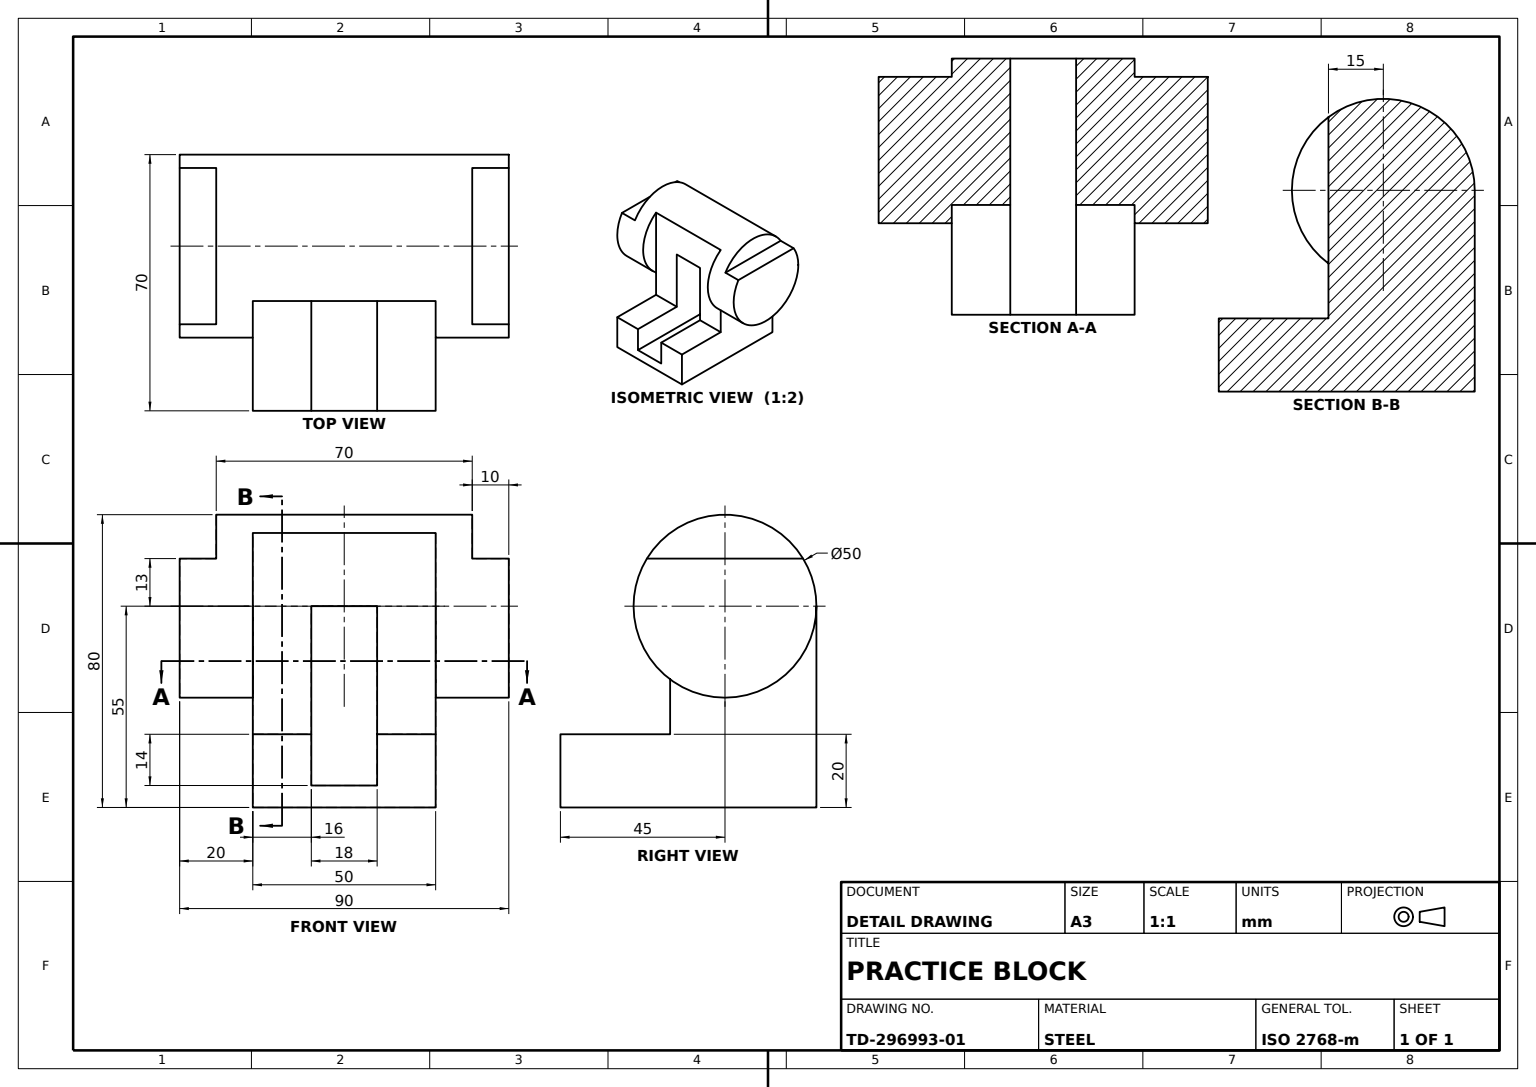
from build123d import *
from build123d.topology import SkipClean

# Parameters (mm, degrees)
U_BASE_DEPTH             = 20
UPRIGHT_WEB_DEPTH        = 50
CYLINDER_50_SKETCH_R     = 25
CYLINDER_50_DEPTH        = 50
WEB_CLEARANCE_CUT_DEPTH  = 50
SIDE_RELIEF_CUT_SKETCH_W = 18
SIDE_RELIEF_CUT_SKETCH_H = 35
SIDE_RELIEF_CUT_DEPTH    = 50
BASE_SLOT_CUT_SKETCH_W   = 50
BASE_SLOT_CUT_SKETCH_H   = 50
BASE_SLOT_CUT_DEPTH      = 10
WEB_SLOT_CUT_SKETCH_W    = 5
WEB_SLOT_CUT_SKETCH_H    = 50
WEB_SLOT_CUT_DEPTH       = 10
END_START                = 20
END_BOSS_A_SKETCH_R      = 25
END_BOSS_A_50_DEPTH      = 20
END_BOSS_B_SKETCH_R      = 25
END_BOSS_B_50_DEPTH      = 20
END_SLOT_A_DEPTH         = 10
END_START_2              = -10
END_SLOT_B_DEPTH         = 10


with BuildPart() as part:
    # U Base Profile Sketch → U Base (new body)
    with BuildSketch(Plane(origin=(0, 0, 0), x_dir=(0, 0, -1), z_dir=(1, 0, 0))):
        Polygon((25, 0), (-25, 0), (-25, 20), (-9, 20), (-9, 6), (9, 6), (9, 20), (25, 20), align=None)
    extrude(amount=U_BASE_DEPTH)

    # Upright Web Sketch → Upright Web (add)
    with BuildSketch(Plane.ZY):
        Polygon((-9, 20), (-9, 65), (9, 65), (9, 20), (25, 20), (25, 70), (-25, 70), (-25, 20), align=None)
        Polygon((25, 20), (9, 20), (9, 6), (-9, 6), (-9, 20), (-25, 20), (-25, 0), (25, 0), align=None)
    extrude(amount=UPRIGHT_WEB_DEPTH)

    # Cylinder Ø50 Sketch → Cylinder Ø50 (add)
    with BuildSketch(Plane.XY.offset(25)):
        with Locations((-25, 55)):
            Circle(CYLINDER_50_SKETCH_R)
    extrude(amount=-CYLINDER_50_DEPTH)

    # Web Clearance Cut Sketch → Web Clearance Cut (cut)
    with SkipClean():  # the faces are left unmerged after this step: merging them gives an invalid solid
        with BuildSketch(Plane.XY.offset(25)):
            with BuildLine():
                Line((-50, 70), (-50, 55))
                ThreePointArc((-50, 55), (-48.717082, 62.905694), (-45, 70))
                Line((-45, 70), (-50, 70))
            make_face()
            with BuildLine():
                ThreePointArc((-5, 70), (-1.282918, 62.905694), (0, 55))
                Line((0, 55), (0, 70))
                Line((0, 70), (-5, 70))
            make_face()
        extrude(amount=-WEB_CLEARANCE_CUT_DEPTH, mode=Mode.SUBTRACT)

    # Side Relief Cut Sketch → Side Relief Cut (cut)
    with SkipClean():  # the faces are left unmerged after this step: merging them gives an invalid solid
        with BuildSketch(Plane(origin=(0, 0, 0), x_dir=(0, 0, -1), z_dir=(1, 0, 0))):
            with Locations((0, 37.5)):
                Rectangle(SIDE_RELIEF_CUT_SKETCH_W, SIDE_RELIEF_CUT_SKETCH_H)
        extrude(amount=-SIDE_RELIEF_CUT_DEPTH, mode=Mode.SUBTRACT)

    # Base Slot Cut Sketch → Base Slot Cut (cut)
    with SkipClean():  # the faces are left unmerged after this step: merging them gives an invalid solid
        with BuildSketch(Plane(origin=(0, 0, 0), x_dir=(0, 0, -1), z_dir=(1, 0, 0))):
            with Locations((0, 45)):
                Rectangle(BASE_SLOT_CUT_SKETCH_W, BASE_SLOT_CUT_SKETCH_H)
        extrude(amount=-BASE_SLOT_CUT_DEPTH, mode=Mode.SUBTRACT)

    # Web Slot Cut Sketch → Web Slot Cut (cut)
    with SkipClean():  # the faces are left unmerged after this step: merging them gives an invalid solid
        with BuildSketch(Plane.XZ.offset(-70)):
            with Locations((-7.5, 0)):
                Rectangle(WEB_SLOT_CUT_SKETCH_W, WEB_SLOT_CUT_SKETCH_H)
        extrude(amount=-WEB_SLOT_CUT_DEPTH, mode=Mode.SUBTRACT)

    # End Boss A Sketch → End Boss A Ø50 (add)
    with BuildSketch(Plane.XY.offset(25).offset(END_START)):
        with Locations((-25, 55)):
            Circle(END_BOSS_A_SKETCH_R)
    extrude(amount=-END_BOSS_A_50_DEPTH)

    # End Boss B Sketch → End Boss B Ø50 (add)
    with BuildSketch(Plane(origin=(0, 0, -25), x_dir=(-1, 0, 0), z_dir=(0, 0, -1))):
        with Locations(Location((25, 55, 0), (0, 0, 180))):
            Circle(END_BOSS_B_SKETCH_R)
    extrude(amount=END_BOSS_B_50_DEPTH)

    # End Slot A Sketch → End Slot A (cut)
    with BuildSketch(Plane.XY.offset(45)):
        with BuildLine():
            Line((-46.354157, 68), (-3.645843, 68))
            ThreePointArc((-3.645843, 68), (-25, 80), (-46.354157, 68))
        make_face()
    extrude(amount=-END_SLOT_A_DEPTH, mode=Mode.SUBTRACT)

    # End Slot B Sketch → End Slot B (cut)
    with BuildSketch(Plane(origin=(0, 0, -45), x_dir=(-1, 0, 0), z_dir=(0, 0, -1)).offset(END_START_2)):
        with BuildLine():
            Line((3.645843, 68), (46.354157, 68))
            ThreePointArc((46.354157, 68), (25, 80), (3.645843, 68))
        make_face()
    extrude(amount=END_SLOT_B_DEPTH, mode=Mode.SUBTRACT)


solid = part.part
